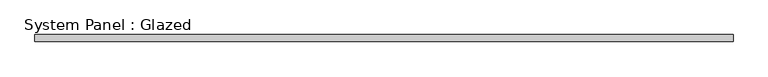
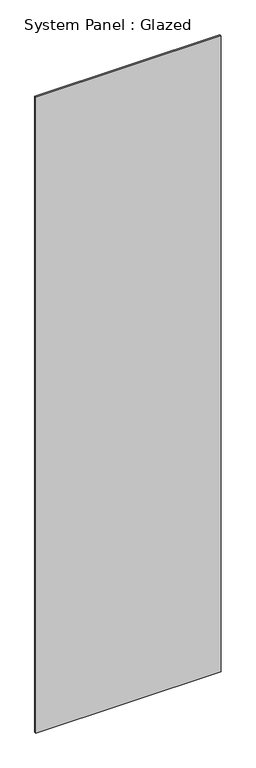
"""IFC4 building model written with IfcOpenShell, lengths in millimetres: plate geometry, System Panel : Glazed."""

from ifc_helpers import new_model, si_unit, origin, origin_with_axes, place, context, project, spatial, polyline, outline, extrude, source, transform, mapped, element, save


def system_panel_glazed_3d5b17eb(model_context):
    return source(origin(), model_context, "Body", "SweptSolid", [
        extrude(outline(polyline([(1259.3594942, 19.05), (-1259.3594942, 19.05), (-1259.3594942, 44.45), (1259.3594942, 44.45), (1259.3594942, 19.05)])), origin_with_axes(), (0.0, 0.0, 1.0), 9144.0),
    ])


if __name__ == "__main__":
    model = new_model("IFC4")
    model_context = context("Model", 3, world=origin())
    ifc_project = project(units=[si_unit("LENGTHUNIT", "METRE", prefix="MILLI")], contexts=[model_context])
    site = spatial("IfcSite", under=ifc_project)
    building = spatial("IfcBuilding", under=site)
    placement = place(None, origin())
    system_panel_glazed_shape = system_panel_glazed_3d5b17eb(model_context)
    element("IfcPlate", 1, ObjectType="System Panel : Glazed", at=placement, inside=building, context=model_context, shape_type="MappedRepresentation", body=[
        mapped(system_panel_glazed_shape, transform((0.0, 0.0, 0.0), x_axis=(1.0, 0.0, 0.0), y_axis=(0.0, 1.0, 0.0), z_axis=(0.0, 0.0, 1.0))),
    ])
    save(model, "model.ifc")

# Revit data of these elements
# Type "System Panel : Glazed"
#   Construction Type Id = "GSP4R"
#   Analytic Construction = "1/8 in Pilkington single glazing"
#   Visual Light Transmittance = 0.9
#   Solar Heat Gain Coefficient = 0.86
#   Heat Transfer Coefficient (U) = 1.18115 BTU/(h·ft²·°F)
#   Define Thermal Properties by = 1
# Element 1 (IfcPlate, "System Panel : Glazed")
#   Materials on its faces: "Glass"
# Materials
#   "Glass": class "Glass", colour RGB 0 128 192, transparency 0.75, Description = "Soda Lime Glass", Cost = 0
